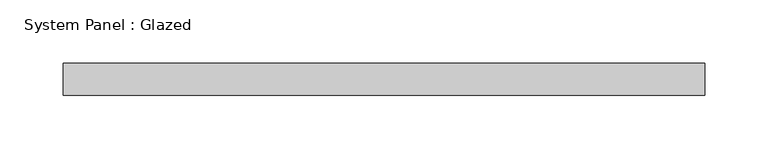
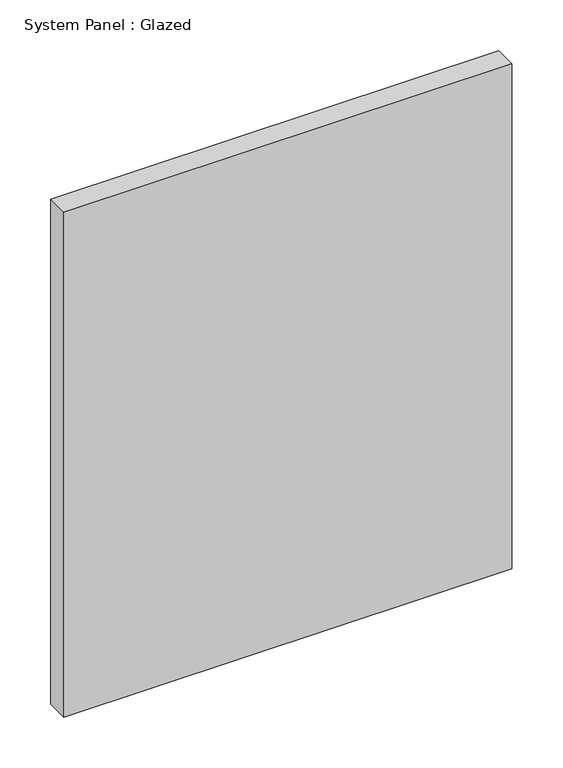
"""IFC4 building model written with IfcOpenShell, lengths in millimetres: plate geometry, System Panel : Glazed."""

from ifc_helpers import new_model, si_unit, origin, origin_with_axes, place, context, project, spatial, polyline, outline, extrude, source, transform, mapped, element, save


def system_panel_glazed_618baec5(model_context):
    return source(origin(), model_context, "Body", "SweptSolid", [
        extrude(outline(polyline([(254.0, 19.05), (-254.0, 19.05), (-254.0, 44.45), (254.0, 44.45), (254.0, 19.05)])), origin_with_axes(), (0.0, 0.0, 1.0), 605.2147936),
    ])


if __name__ == "__main__":
    model = new_model("IFC4")
    model_context = context("Model", 3, world=origin())
    ifc_project = project(units=[si_unit("LENGTHUNIT", "METRE", prefix="MILLI")], contexts=[model_context])
    site = spatial("IfcSite", under=ifc_project)
    building = spatial("IfcBuilding", under=site)
    placement = place(None, origin())
    system_panel_glazed_shape = system_panel_glazed_618baec5(model_context)
    element("IfcPlate", 1, ObjectType="System Panel : Glazed", at=placement, inside=building, context=model_context, shape_type="MappedRepresentation", body=[
        mapped(system_panel_glazed_shape, transform((0.0, 0.0, 0.0), x_axis=(1.0, 0.0, 0.0), y_axis=(0.0, 1.0, 0.0), z_axis=(0.0, 0.0, 1.0))),
    ])
    save(model, "model.ifc")

# Revit data of these elements
# Type "System Panel : Glazed"
#   Construction Type Id = "GSP4R"
#   Analytic Construction = "1/8 in Pilkington single glazing"
#   Visual Light Transmittance = 0.9
#   Solar Heat Gain Coefficient = 0.86
#   Heat Transfer Coefficient (U) = 1.18115 BTU/(h·ft²·°F)
#   Define Thermal Properties by = 1
# Element 1 (IfcPlate, "System Panel : Glazed")
#   Materials on its faces: "Glass"
# Materials
#   "Glass": class "Glass", colour RGB 0 128 192, transparency 0.75, Description = "Soda Lime Glass", Cost = 0
